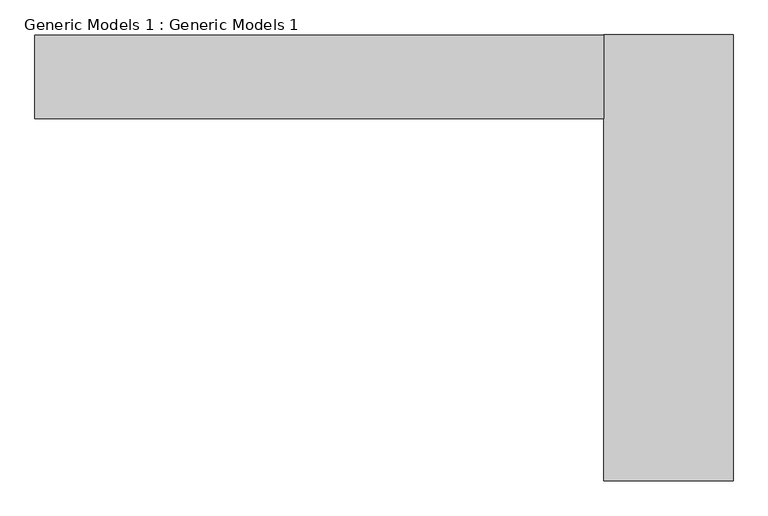
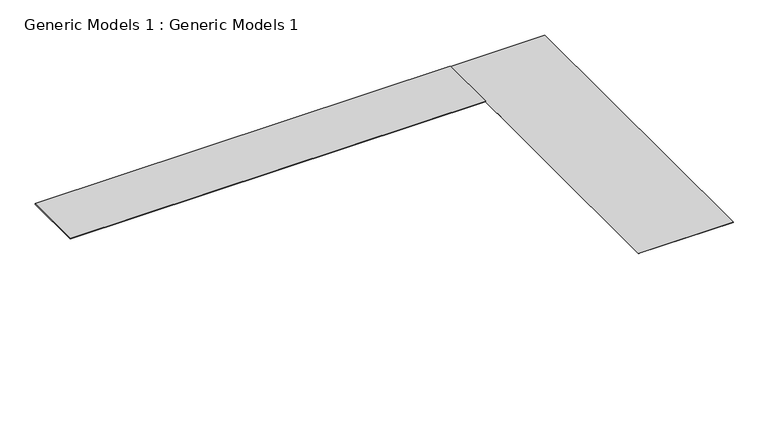
"""IFC4 building model written with IfcOpenShell, lengths in millimetres: proxy geometry, Generic Models 1 : Generic Models 1."""

from ifc_helpers import new_model, si_unit, frame, origin, place, context, project, spatial, polyline, outline, extrude, source, transform, mapped, element, save


def generic_models_1_generic_models_1_fe68cf6e(model_context):
    return source(origin(), model_context, "Body", "SweptSolid", [
        extrude(outline(polyline([(18814.4038118, 19698.2107351), (-17987.1489856, 19698.2107351), (-17987.1489856, 25092.2590425), (18814.4038118, 25092.2590425), (18814.4038118, 19698.2107351)])), frame((0.0, 0.0, -914.4), z_axis=(0.0, 0.0, 1.0), x_axis=(1.0, 0.0, 0.0)), (0.0, 0.0, 1.0), 62.860383),
        extrude(outline(polyline([(27199.4510144, 25109.355505), (27199.4510144, -3770.444495), (18814.4038118, -3770.444495), (18814.4038118, 25109.355505), (27199.4510144, 25109.355505)])), frame((0.0, 0.0, -914.4), z_axis=(0.0, 0.0, 1.0), x_axis=(1.0, 0.0, 0.0)), (0.0, 0.0, 1.0), 29.9349183),
    ])


if __name__ == "__main__":
    model = new_model("IFC4")
    model_context = context("Model", 3, world=origin())
    ifc_project = project(units=[si_unit("LENGTHUNIT", "METRE", prefix="MILLI")], contexts=[model_context])
    site = spatial("IfcSite", under=ifc_project)
    building = spatial("IfcBuilding", under=site)
    placement = place(None, origin())
    generic_models_1_generic_models_1_shape = generic_models_1_generic_models_1_fe68cf6e(model_context)
    element("IfcBuildingElementProxy", 1, Name="Generic Models 1 : Generic Models 1", ObjectType="Generic Models 1 : Generic Models 1", at=placement, inside=building, context=model_context, shape_type="MappedRepresentation", body=[
        mapped(generic_models_1_generic_models_1_shape, transform((0.0, 0.0, 0.0), x_axis=(1.0, 0.0, 0.0), y_axis=(0.0, 1.0, 0.0), z_axis=(0.0, 0.0, 1.0))),
    ])
    save(model, "model.ifc")
